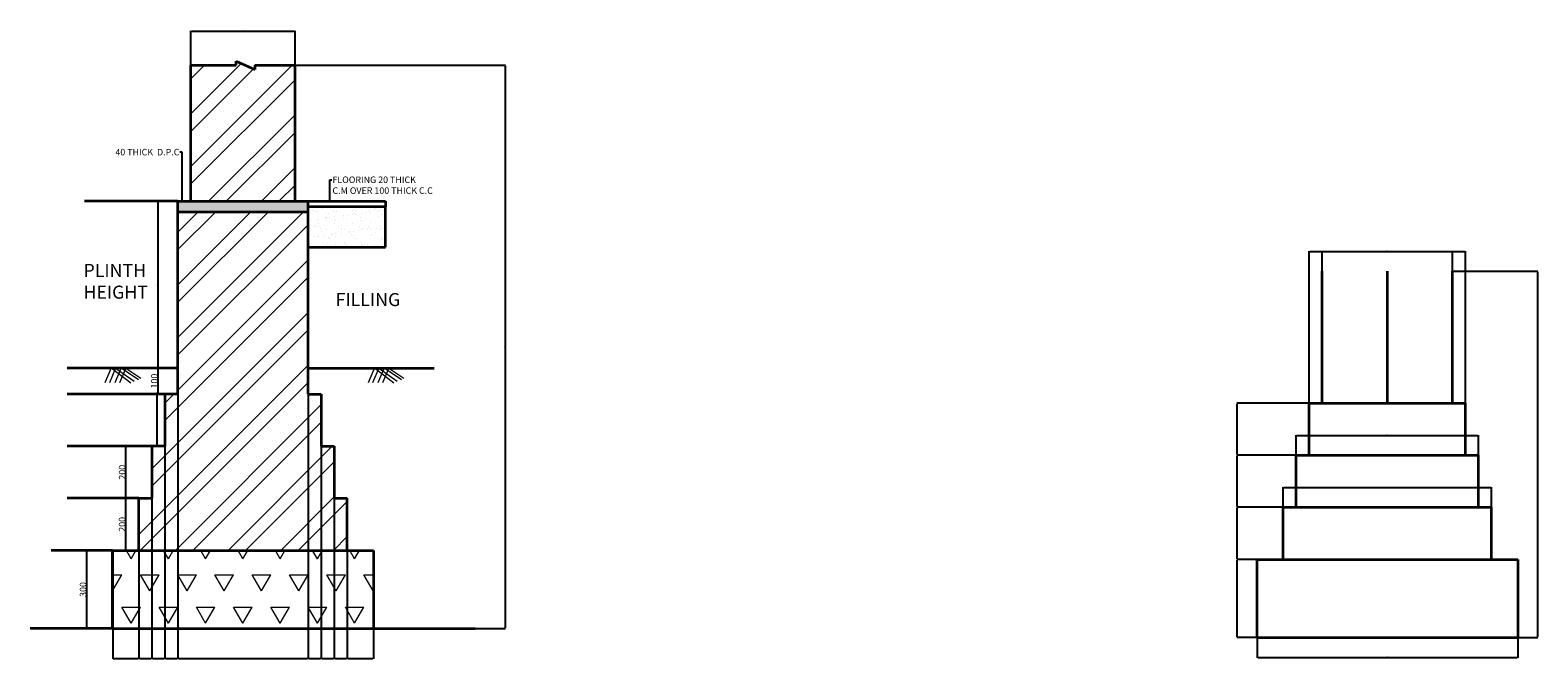
# Model space of a CAD drawing. Units: millimetres. Extents: x 31035 to 42175, y 1348 to 3924.
# Tile 2 of 2: x 36392 to 42175, y 1348 to 3761. Entities that reach past the tile are written whole.
import ezdxf
from ezdxf import colors
from ezdxf.entities.mleader import LeaderData, LeaderLine
from ezdxf.math import Vec2, Vec3

# ---------------------------------------------------------------- set-up
doc = ezdxf.new("R2010")
doc.units = ezdxf.units.MM
for name, color, linetype, lineweight in [('A-ANNO-DIMS', 2, 'Continuous', 18), ('A-ANNO-SYMB', 3, 'Continuous', 18), ('A-ANNO-TEXT', 7, 'Continuous', 18), ('A-SECT', 7, 'Continuous', 35), ('A-WALL-PATT', 8, 'Continuous', 13), ('C-TOPO-PATT', 9, 'Continuous', 13), ('S-FNDN-PATT', 252, 'Continuous', 13)]:
    doc.layers.add(name, color=color, linetype=linetype, lineweight=lineweight)
doc.styles.get("Standard").update_dxf_attribs({"font": 'arial.ttf'})
doc.dimstyles.new('ISO-25', dxfattribs={"dimtxt": 2.5, "dimasz": 2.5, "dimexe": 1.25, "dimexo": 0.625, "dimtad": 1, "dimtxsty": 'Standard', "dimcen": 2.5, "dimadec": 0, "dimazin": 0, "dimtfac": 1, "dimtmove": 0, "dimatfit": 3, "dimfxl": 1, "dimarcsym": 0})
pattern_1 = [(45, (28921.22, 0), (-101.0279, 101.0279), []), (45, (28988.58, 0), (-101.0279, 101.0279), [])]

# ---------------------------------------------------------------- blocks, each defined once
blk = doc.blocks.new('*D15')
at = {"layer": 'A-ANNO-DIMS', "color": 0, "lineweight": -2, "transparency": 16777216}
for p, q in [((36828.2, 3104.1), (36882.5, 3104.1)), ((36881.2, 3101.6), (36881.2, 2466.6)), ((36828.2, 2464.1), (36882.5, 2464.1))]:
    blk.add_line(p, q, dxfattribs=at)
at = {"layer": 'A-ANNO-DIMS', "color": 0, "transparency": 16777216}
for points in [[(36880.8, 3101.6), (36881.7, 3101.6), (36881.2, 3104.1)], [(36880.8, 2466.6), (36881.7, 2466.6), (36881.2, 2464.1)]]:
    blk.add_solid(points, dxfattribs=at)
at = {"layer": 'Defpoints', "color": 0, "transparency": 16777216}
for p in [(36827.6, 3104.1), (36827.6, 2464.1), (36881.2, 2464.1)]:
    blk.add_point(p, dxfattribs=at)
at = {"layer": 'A-ANNO-DIMS', "color": 0, "transparency": 16777216, "insert": (36879.3, 2784.1), "char_height": 2.5, "attachment_point": 5, "rotation": 90}
blk.add_mtext('640', dxfattribs=at)
blk = doc.blocks.new('*D16')
at = {"layer": 'A-ANNO-DIMS', "color": 0, "lineweight": -2, "transparency": 16777216}
for p, q in [((36881.4, 2461.6), (36881.4, 2366.6)), ((36881.9, 2464.1), (36882.7, 2464.1)), ((36881.9, 2364.1), (36882.7, 2364.1))]:
    blk.add_line(p, q, dxfattribs=at)
at = {"layer": 'A-ANNO-DIMS', "color": 0, "transparency": 16777216}
for points in [[(36881, 2461.6), (36881.9, 2461.6), (36881.4, 2464.1)], [(36881, 2366.6), (36881.9, 2366.6), (36881.4, 2364.1)]]:
    blk.add_solid(points, dxfattribs=at)
at = {"layer": 'Defpoints', "color": 0, "transparency": 16777216}
for p in [(36881.2, 2464.1), (36881.2, 2364.1), (36881.4, 2364.1)]:
    blk.add_point(p, dxfattribs=at)
at = {"layer": 'A-ANNO-DIMS', "color": 0, "transparency": 16777216, "insert": (36868.1, 2414.1), "char_height": 2.5, "attachment_point": 5, "rotation": 90}
blk.add_mtext('{\\H10x;100}', dxfattribs=at)
blk = doc.blocks.new('*D17')
at = {"layer": 'A-ANNO-DIMS', "color": 0, "lineweight": -2, "transparency": 16777216}
for p, q in [((36881.2, 2366.6), (36876.9, 2366.6)), ((36878.2, 2364.1), (36878.2, 2166.6)), ((36881.2, 2164.1), (36876.9, 2164.1))]:
    blk.add_line(p, q, dxfattribs=at)
at = {"layer": 'A-ANNO-DIMS', "color": 0, "transparency": 16777216}
for points in [[(36877.7, 2364.1), (36878.6, 2364.1), (36878.2, 2366.6)], [(36877.7, 2166.6), (36878.6, 2166.6), (36878.2, 2164.1)]]:
    blk.add_solid(points, dxfattribs=at)
at = {"layer": 'Defpoints', "color": 0, "transparency": 16777216}
for p in [(36881.9, 2366.6), (36878.2, 2164.1), (36881.9, 2164.1)]:
    blk.add_point(p, dxfattribs=at)
at = {"layer": 'A-ANNO-DIMS', "color": 0, "transparency": 16777216, "insert": (36876, 2265.3), "char_height": 2.5, "attachment_point": 5, "rotation": 90}
blk.add_mtext('202,5', dxfattribs=at)
blk = doc.blocks.new('*D18')
at = {"layer": 'A-ANNO-DIMS', "color": 0, "lineweight": -2, "transparency": 16777216}
for p, q in [((36758.3, 2161.6), (36758.3, 1966.6)), ((36758.9, 2164.1), (36759.5, 2164.1)), ((36758.9, 1964.1), (36759.5, 1964.1))]:
    blk.add_line(p, q, dxfattribs=at)
at = {"layer": 'A-ANNO-DIMS', "color": 0, "transparency": 16777216}
for points in [[(36757.8, 2161.6), (36758.7, 2161.6), (36758.3, 2164.1)], [(36757.8, 1966.6), (36758.7, 1966.6), (36758.3, 1964.1)]]:
    blk.add_solid(points, dxfattribs=at)
at = {"layer": 'Defpoints', "color": 0, "transparency": 16777216}
for p in [(36758.3, 2164.1), (36758.3, 1964.1), (36758.3, 1964.1)]:
    blk.add_point(p, dxfattribs=at)
at = {"layer": 'A-ANNO-DIMS', "color": 0, "transparency": 16777216, "insert": (36744.9, 2064.1), "char_height": 2.5, "attachment_point": 5, "rotation": 90}
blk.add_mtext('{\\H10x;200}', dxfattribs=at)
blk = doc.blocks.new('*D19')
at = {"layer": 'A-ANNO-DIMS', "color": 0, "lineweight": -2, "transparency": 16777216}
for p, q in [((36758.9, 1964.1), (36757, 1964.1)), ((36758.2, 1961.6), (36758.2, 1766.6)), ((36758.9, 1764.1), (36757, 1764.1))]:
    blk.add_line(p, q, dxfattribs=at)
at = {"layer": 'A-ANNO-DIMS', "color": 0, "transparency": 16777216}
for points in [[(36757.8, 1961.6), (36758.6, 1961.6), (36758.2, 1964.1)], [(36757.8, 1766.6), (36758.6, 1766.6), (36758.2, 1764.1)]]:
    blk.add_solid(points, dxfattribs=at)
at = {"layer": 'Defpoints', "color": 0, "transparency": 16777216}
for p in [(36759.5, 1964.1), (36758.2, 1764.1), (36759.5, 1764.1)]:
    blk.add_point(p, dxfattribs=at)
at = {"layer": 'A-ANNO-DIMS', "color": 0, "transparency": 16777216, "insert": (36744.8, 1864.1), "char_height": 2.5, "attachment_point": 5, "rotation": 90}
blk.add_mtext('{\\H10x;200}', dxfattribs=at)
blk = doc.blocks.new('*D20')
at = {"layer": 'A-ANNO-DIMS', "color": 0, "lineweight": -2, "transparency": 16777216}
for p, q in [((36631.4, 1764.1), (36607.1, 1764.1)), ((36608.3, 1761.6), (36608.3, 1466.6)), ((36631.4, 1464.1), (36607.1, 1464.1))]:
    blk.add_line(p, q, dxfattribs=at)
at = {"layer": 'A-ANNO-DIMS', "color": 0, "transparency": 16777216}
for points in [[(36607.9, 1761.6), (36608.7, 1761.6), (36608.3, 1764.1)], [(36607.9, 1466.6), (36608.7, 1466.6), (36608.3, 1464.1)]]:
    blk.add_solid(points, dxfattribs=at)
at = {"layer": 'Defpoints', "color": 0, "transparency": 16777216}
for p in [(36632, 1764.1), (36608.3, 1464.1), (36632, 1464.1)]:
    blk.add_point(p, dxfattribs=at)
at = {"layer": 'A-ANNO-DIMS', "color": 0, "transparency": 16777216, "insert": (36594.9, 1614.1), "char_height": 2.5, "attachment_point": 5, "rotation": 90}
blk.add_mtext('{\\H10x;300}', dxfattribs=at)
blk = doc.blocks.new('EARTH-SYMBOL-B')
for p, q in [((24.2, 58), (0, 0.7)), ((24.2, 58), (99.5, 0.7)), ((61.9, 58), (37.7, 0.7)), ((61.9, 58), (128.5, 13.8)), ((40.9, 57.3), (16.7, 0)), ((40.9, 57.3), (111.8, 6.5)), ((80.1, 57.3), (55.9, 0)), ((80.1, 57.3), (137.9, 18.1))]:
    blk.add_line(p, q)
blk = doc.blocks.new('*D26')
at = {"layer": 'A-ANNO-DIMS', "color": 0, "lineweight": -2, "transparency": 16777216}
for p, q in [((37409.1, 3626.5), (38214.9, 3626.5)), ((38213.7, 3624), (38213.7, 1466.6)), ((37709.1, 1464.1), (38214.9, 1464.1))]:
    blk.add_line(p, q, dxfattribs=at)
at = {"layer": 'A-ANNO-DIMS', "color": 0, "transparency": 16777216}
for points in [[(38213.3, 3624), (38214.1, 3624), (38213.7, 3626.5)], [(38213.3, 1466.6), (38214.1, 1466.6), (38213.7, 1464.1)]]:
    blk.add_solid(points, dxfattribs=at)
at = {"layer": 'Defpoints', "color": 0, "transparency": 16777216}
for p in [(37408.5, 3626.5), (37708.5, 1464.1), (38213.7, 1464.1)]:
    blk.add_point(p, dxfattribs=at)
at = {"layer": 'A-ANNO-DIMS', "color": 0, "transparency": 16777216, "insert": (38211.8, 2545.3), "char_height": 2.5, "attachment_point": 5, "rotation": 90}
blk.add_mtext('2162.4', dxfattribs=at)
blk = doc.blocks.new('*D27')
at = {"layer": 'A-ANNO-DIMS', "color": 0, "lineweight": -2, "transparency": 16777216}
for p, q in [((37008.5, 3627.2), (37008.5, 3758.8)), ((37011, 3757.5), (37406, 3757.5)), ((37408.5, 3627.2), (37408.5, 3758.8))]:
    blk.add_line(p, q, dxfattribs=at)
at = {"layer": 'A-ANNO-DIMS', "color": 0, "transparency": 16777216}
for points in [[(37011, 3757.9), (37011, 3757.1), (37008.5, 3757.5)], [(37406, 3757.9), (37406, 3757.1), (37408.5, 3757.5)]]:
    blk.add_solid(points, dxfattribs=at)
at = {"layer": 'Defpoints', "color": 0, "transparency": 16777216}
for p in [(37408.5, 3757.5), (37008.5, 3626.5), (37408.5, 3626.5)]:
    blk.add_point(p, dxfattribs=at)
at = {"layer": 'A-ANNO-DIMS', "color": 0, "transparency": 16777216, "insert": (37208.5, 3759.4), "char_height": 2.5, "attachment_point": 5}
blk.add_mtext('400', dxfattribs=at)
blk = doc.blocks.new('*D28')
at = {"layer": 'A-ANNO-DIMS', "color": 0, "lineweight": -2, "transparency": 16777216}
for p, q in [((41098.1, 1429), (41098.1, 1352.4)), ((42098.1, 1429), (42098.1, 1352.4)), ((41100.6, 1353.6), (42095.6, 1353.6))]:
    blk.add_line(p, q, dxfattribs=at)
at = {"layer": 'A-ANNO-DIMS', "color": 0, "transparency": 16777216}
for points in [[(41100.6, 1354.1), (41100.6, 1353.2), (41098.1, 1353.6)], [(42095.6, 1354.1), (42095.6, 1353.2), (42098.1, 1353.6)]]:
    blk.add_solid(points, dxfattribs=at)
at = {"layer": 'Defpoints', "color": 0, "transparency": 16777216}
for p in [(41098.1, 1429.6), (42098.1, 1429.6), (42098.1, 1353.6)]:
    blk.add_point(p, dxfattribs=at)
at = {"layer": 'A-ANNO-DIMS', "color": 0, "transparency": 16777216, "insert": (41598.1, 1355.5), "char_height": 2.5, "attachment_point": 5}
blk.add_mtext('1000', dxfattribs=at)
blk = doc.blocks.new('*D29')
at = {"layer": 'A-ANNO-DIMS', "color": 0, "lineweight": -2, "transparency": 16777216}
for p, q in [((41348.1, 2836.6), (41348.1, 2913.2)), ((41350.6, 2911.9), (41845.6, 2911.9)), ((41848.1, 2836.6), (41848.1, 2913.2))]:
    blk.add_line(p, q, dxfattribs=at)
at = {"layer": 'A-ANNO-DIMS', "color": 0, "transparency": 16777216}
for points in [[(41350.6, 2912.3), (41350.6, 2911.5), (41348.1, 2911.9)], [(41845.6, 2912.3), (41845.6, 2911.5), (41848.1, 2911.9)]]:
    blk.add_solid(points, dxfattribs=at)
at = {"layer": 'Defpoints', "color": 0, "transparency": 16777216}
for p in [(41848.1, 2911.9), (41348.1, 2835.9), (41848.1, 2835.9)]:
    blk.add_point(p, dxfattribs=at)
at = {"layer": 'A-ANNO-DIMS', "color": 0, "transparency": 16777216, "insert": (41598.1, 2913.8), "char_height": 2.5, "attachment_point": 5}
blk.add_mtext('500', dxfattribs=at)
blk = doc.blocks.new('*D30')
at = {"layer": 'A-ANNO-DIMS', "color": 0, "lineweight": -2, "transparency": 16777216}
for p, q in [((41097.5, 1729.6), (41020.8, 1729.6)), ((41022.1, 1432.1), (41022.1, 1727.1)), ((41097.5, 1429.6), (41020.8, 1429.6))]:
    blk.add_line(p, q, dxfattribs=at)
at = {"layer": 'A-ANNO-DIMS', "color": 0, "transparency": 16777216}
for points in [[(41021.7, 1727.1), (41022.5, 1727.1), (41022.1, 1729.6)], [(41021.7, 1432.1), (41022.5, 1432.1), (41022.1, 1429.6)]]:
    blk.add_solid(points, dxfattribs=at)
at = {"layer": 'Defpoints', "color": 0, "transparency": 16777216}
for p in [(41022.1, 1729.6), (41098.1, 1729.6), (41098.1, 1429.6)]:
    blk.add_point(p, dxfattribs=at)
at = {"layer": 'A-ANNO-DIMS', "color": 0, "transparency": 16777216, "insert": (41020.2, 1579.6), "char_height": 2.5, "attachment_point": 5, "rotation": 90}
blk.add_mtext('300', dxfattribs=at)
blk = doc.blocks.new('*D31')
at = {"layer": 'A-ANNO-DIMS', "color": 0, "lineweight": -2, "transparency": 16777216}
for p, q in [((41197.5, 1929.6), (41020.8, 1929.6)), ((41022.1, 1732.1), (41022.1, 1927.1)), ((41197.5, 1729.6), (41020.8, 1729.6))]:
    blk.add_line(p, q, dxfattribs=at)
at = {"layer": 'A-ANNO-DIMS', "color": 0, "transparency": 16777216}
for points in [[(41021.7, 1927.1), (41022.5, 1927.1), (41022.1, 1929.6)], [(41021.7, 1732.1), (41022.5, 1732.1), (41022.1, 1729.6)]]:
    blk.add_solid(points, dxfattribs=at)
at = {"layer": 'Defpoints', "color": 0, "transparency": 16777216}
for p in [(41022.1, 1929.6), (41198.1, 1929.6), (41198.1, 1729.6)]:
    blk.add_point(p, dxfattribs=at)
at = {"layer": 'A-ANNO-DIMS', "color": 0, "transparency": 16777216, "insert": (41020.2, 1829.6), "char_height": 2.5, "attachment_point": 5, "rotation": 90}
blk.add_mtext('200', dxfattribs=at)
blk = doc.blocks.new('*D32')
at = {"layer": 'A-ANNO-DIMS', "color": 0, "lineweight": -2, "transparency": 16777216}
for p, q in [((41247.5, 2129.6), (41020.8, 2129.6)), ((41022.1, 1932.1), (41022.1, 2127.1)), ((41247.5, 1929.6), (41020.8, 1929.6))]:
    blk.add_line(p, q, dxfattribs=at)
at = {"layer": 'A-ANNO-DIMS', "color": 0, "transparency": 16777216}
for points in [[(41021.7, 2127.1), (41022.5, 2127.1), (41022.1, 2129.6)], [(41021.7, 1932.1), (41022.5, 1932.1), (41022.1, 1929.6)]]:
    blk.add_solid(points, dxfattribs=at)
at = {"layer": 'Defpoints', "color": 0, "transparency": 16777216}
for p in [(41022.1, 2129.6), (41248.1, 2129.6), (41248.1, 1929.6)]:
    blk.add_point(p, dxfattribs=at)
at = {"layer": 'A-ANNO-DIMS', "color": 0, "transparency": 16777216, "insert": (41020.2, 2029.6), "char_height": 2.5, "attachment_point": 5, "rotation": 90}
blk.add_mtext('200', dxfattribs=at)
blk = doc.blocks.new('*D33')
at = {"layer": 'A-ANNO-DIMS', "color": 0, "lineweight": -2, "transparency": 16777216}
for p, q in [((41297.5, 2329.6), (41020.8, 2329.6)), ((41022.1, 2132.1), (41022.1, 2327.1)), ((41297.5, 2129.6), (41020.8, 2129.6))]:
    blk.add_line(p, q, dxfattribs=at)
at = {"layer": 'A-ANNO-DIMS', "color": 0, "transparency": 16777216}
for points in [[(41021.7, 2327.1), (41022.5, 2327.1), (41022.1, 2329.6)], [(41021.7, 2132.1), (41022.5, 2132.1), (41022.1, 2129.6)]]:
    blk.add_solid(points, dxfattribs=at)
at = {"layer": 'Defpoints', "color": 0, "transparency": 16777216}
for p in [(41022.1, 2329.6), (41298.1, 2329.6), (41298.1, 2129.6)]:
    blk.add_point(p, dxfattribs=at)
at = {"layer": 'A-ANNO-DIMS', "color": 0, "transparency": 16777216, "insert": (41020.2, 2229.6), "char_height": 2.5, "attachment_point": 5, "rotation": 90}
blk.add_mtext('200', dxfattribs=at)
blk = doc.blocks.new('*D34')
at = {"layer": 'A-ANNO-DIMS', "color": 0, "lineweight": -2, "transparency": 16777216}
for p, q in [((41198.1, 1930.3), (41198.1, 2006.9)), ((41200.6, 2005.6), (41995.6, 2005.6)), ((41998.1, 1930.3), (41998.1, 2006.9))]:
    blk.add_line(p, q, dxfattribs=at)
at = {"layer": 'A-ANNO-DIMS', "color": 0, "transparency": 16777216}
for points in [[(41200.6, 2006.1), (41200.6, 2005.2), (41198.1, 2005.6)], [(41995.6, 2006.1), (41995.6, 2005.2), (41998.1, 2005.6)]]:
    blk.add_solid(points, dxfattribs=at)
at = {"layer": 'Defpoints', "color": 0, "transparency": 16777216}
for p in [(41998.1, 2005.6), (41198.1, 1929.6), (41998.1, 1929.6)]:
    blk.add_point(p, dxfattribs=at)
at = {"layer": 'A-ANNO-DIMS', "color": 0, "transparency": 16777216, "insert": (41598.1, 2007.5), "char_height": 2.5, "attachment_point": 5}
blk.add_mtext('800', dxfattribs=at)
blk = doc.blocks.new('*D35')
at = {"layer": 'A-ANNO-DIMS', "color": 0, "lineweight": -2, "transparency": 16777216}
for p, q in [((41248.1, 2130.3), (41248.1, 2206.9)), ((41250.6, 2205.6), (41945.6, 2205.6)), ((41948.1, 2130.3), (41948.1, 2206.9))]:
    blk.add_line(p, q, dxfattribs=at)
at = {"layer": 'A-ANNO-DIMS', "color": 0, "transparency": 16777216}
for points in [[(41250.6, 2206.1), (41250.6, 2205.2), (41248.1, 2205.6)], [(41945.6, 2206.1), (41945.6, 2205.2), (41948.1, 2205.6)]]:
    blk.add_solid(points, dxfattribs=at)
at = {"layer": 'Defpoints', "color": 0, "transparency": 16777216}
for p in [(41948.1, 2205.6), (41248.1, 2129.6), (41948.1, 2129.6)]:
    blk.add_point(p, dxfattribs=at)
at = {"layer": 'A-ANNO-DIMS', "color": 0, "transparency": 16777216, "insert": (41598.1, 2207.5), "char_height": 2.5, "attachment_point": 5}
blk.add_mtext('700', dxfattribs=at)
blk = doc.blocks.new('*D36')
at = {"layer": 'A-ANNO-DIMS', "color": 0, "lineweight": -2, "transparency": 16777216}
for p, q in [((41298.1, 2330.3), (41298.1, 2913.2)), ((41300.6, 2911.9), (41895.6, 2911.9)), ((41898.1, 2330.3), (41898.1, 2913.2))]:
    blk.add_line(p, q, dxfattribs=at)
at = {"layer": 'A-ANNO-DIMS', "color": 0, "transparency": 16777216}
for points in [[(41300.6, 2912.3), (41300.6, 2911.5), (41298.1, 2911.9)], [(41895.6, 2912.3), (41895.6, 2911.5), (41898.1, 2911.9)]]:
    blk.add_solid(points, dxfattribs=at)
at = {"layer": 'Defpoints', "color": 0, "transparency": 16777216}
for p in [(41898.1, 2911.9), (41298.1, 2329.6), (41898.1, 2329.6)]:
    blk.add_point(p, dxfattribs=at)
at = {"layer": 'A-ANNO-DIMS', "color": 0, "transparency": 16777216, "insert": (41598.1, 2913.8), "char_height": 2.5, "attachment_point": 5}
blk.add_mtext('600', dxfattribs=at)
blk = doc.blocks.new('*D37')
at = {"layer": 'A-ANNO-DIMS', "color": 0, "lineweight": -2, "transparency": 16777216}
for p, q in [((41848.7, 2835.9), (42175.3, 2835.9)), ((42174.1, 2833.4), (42174.1, 1432.1)), ((42098.7, 1429.6), (42175.3, 1429.6))]:
    blk.add_line(p, q, dxfattribs=at)
at = {"layer": 'A-ANNO-DIMS', "color": 0, "transparency": 16777216}
for points in [[(42173.7, 2833.4), (42174.5, 2833.4), (42174.1, 2835.9)], [(42173.7, 1432.1), (42174.5, 1432.1), (42174.1, 1429.6)]]:
    blk.add_solid(points, dxfattribs=at)
at = {"layer": 'Defpoints', "color": 0, "transparency": 16777216}
for p in [(41848.1, 2835.9), (42098.1, 1429.6), (42174.1, 1429.6)]:
    blk.add_point(p, dxfattribs=at)
at = {"layer": 'A-ANNO-DIMS', "color": 0, "transparency": 16777216, "insert": (42172.2, 2132.8), "char_height": 2.5, "attachment_point": 5, "rotation": 90}
blk.add_mtext('1406.3', dxfattribs=at)
blk = doc.blocks.new('*D45')
at = {"layer": 'A-ANNO-DIMS', "color": 0, "lineweight": -2, "transparency": 16777216}
for p, q in [((36708.5, 1763.5), (36708.5, 1347.8)), ((36808.5, 1763.5), (36808.5, 1347.8)), ((36711, 1349.1), (36806, 1349.1))]:
    blk.add_line(p, q, dxfattribs=at)
at = {"layer": 'A-ANNO-DIMS', "color": 0, "transparency": 16777216}
for points in [[(36711, 1349.5), (36711, 1348.7), (36708.5, 1349.1)], [(36806, 1349.5), (36806, 1348.7), (36808.5, 1349.1)]]:
    blk.add_solid(points, dxfattribs=at)
at = {"layer": 'Defpoints', "color": 0, "transparency": 16777216}
for p in [(36708.5, 1764.1), (36808.5, 1764.1), (36808.5, 1349.1)]:
    blk.add_point(p, dxfattribs=at)
at = {"layer": 'A-ANNO-DIMS', "color": 0, "transparency": 16777216, "insert": (36758.5, 1351), "char_height": 2.5, "attachment_point": 5}
blk.add_mtext('100', dxfattribs=at)
blk = doc.blocks.new('*D46')
at = {"layer": 'A-ANNO-DIMS', "color": 0, "lineweight": -2, "transparency": 16777216}
for p, q in [((36858.5, 1963.5), (36858.5, 1347.8)), ((36808.5, 1763.5), (36808.5, 1347.8)), ((36811, 1349.1), (36856, 1349.1))]:
    blk.add_line(p, q, dxfattribs=at)
at = {"layer": 'A-ANNO-DIMS', "color": 0, "transparency": 16777216}
for points in [[(36811, 1349.5), (36811, 1348.7), (36808.5, 1349.1)], [(36856, 1349.5), (36856, 1348.7), (36858.5, 1349.1)]]:
    blk.add_solid(points, dxfattribs=at)
at = {"layer": 'Defpoints', "color": 0, "transparency": 16777216}
for p in [(36858.5, 1964.1), (36808.5, 1764.1), (36858.5, 1349.1)]:
    blk.add_point(p, dxfattribs=at)
at = {"layer": 'A-ANNO-DIMS', "color": 0, "transparency": 16777216, "insert": (36833.5, 1351), "char_height": 2.5, "attachment_point": 5}
blk.add_mtext('50', dxfattribs=at)
blk = doc.blocks.new('*D47')
at = {"layer": 'A-ANNO-DIMS', "color": 0, "lineweight": -2, "transparency": 16777216}
for p, q in [((36908.5, 2163.5), (36908.5, 1347.8)), ((36858.5, 1963.5), (36858.5, 1347.8)), ((36861, 1349.1), (36906, 1349.1))]:
    blk.add_line(p, q, dxfattribs=at)
at = {"layer": 'A-ANNO-DIMS', "color": 0, "transparency": 16777216}
for points in [[(36861, 1349.5), (36861, 1348.7), (36858.5, 1349.1)], [(36906, 1349.5), (36906, 1348.7), (36908.5, 1349.1)]]:
    blk.add_solid(points, dxfattribs=at)
at = {"layer": 'Defpoints', "color": 0, "transparency": 16777216}
for p in [(36908.5, 2164.1), (36858.5, 1964.1), (36908.5, 1349.1)]:
    blk.add_point(p, dxfattribs=at)
at = {"layer": 'A-ANNO-DIMS', "color": 0, "transparency": 16777216, "insert": (36883.5, 1351), "char_height": 2.5, "attachment_point": 5}
blk.add_mtext('50', dxfattribs=at)
blk = doc.blocks.new('*D48')
at = {"layer": 'A-ANNO-DIMS', "color": 0, "lineweight": -2, "transparency": 16777216}
for p, q in [((36958.5, 2363.5), (36958.5, 1347.8)), ((36908.5, 2163.5), (36908.5, 1347.8)), ((36911, 1349.1), (36956, 1349.1))]:
    blk.add_line(p, q, dxfattribs=at)
at = {"layer": 'A-ANNO-DIMS', "color": 0, "transparency": 16777216}
for points in [[(36911, 1349.5), (36911, 1348.7), (36908.5, 1349.1)], [(36956, 1349.5), (36956, 1348.7), (36958.5, 1349.1)]]:
    blk.add_solid(points, dxfattribs=at)
at = {"layer": 'Defpoints', "color": 0, "transparency": 16777216}
for p in [(36958.5, 2364.1), (36908.5, 2164.1), (36958.5, 1349.1)]:
    blk.add_point(p, dxfattribs=at)
at = {"layer": 'A-ANNO-DIMS', "color": 0, "transparency": 16777216, "insert": (36933.5, 1351), "char_height": 2.5, "attachment_point": 5}
blk.add_mtext('50', dxfattribs=at)
blk = doc.blocks.new('*D49')
at = {"layer": 'A-ANNO-DIMS', "color": 0, "lineweight": -2, "transparency": 16777216}
for p, q in [((36958.5, 2363.5), (36958.5, 1347.8)), ((37458.5, 2363.5), (37458.5, 1347.8)), ((36961, 1349.1), (37456, 1349.1))]:
    blk.add_line(p, q, dxfattribs=at)
at = {"layer": 'A-ANNO-DIMS', "color": 0, "transparency": 16777216}
for points in [[(36961, 1349.5), (36961, 1348.7), (36958.5, 1349.1)], [(37456, 1349.5), (37456, 1348.7), (37458.5, 1349.1)]]:
    blk.add_solid(points, dxfattribs=at)
at = {"layer": 'Defpoints', "color": 0, "transparency": 16777216}
for p in [(36958.5, 2364.1), (37458.5, 2364.1), (37458.5, 1349.1)]:
    blk.add_point(p, dxfattribs=at)
at = {"layer": 'A-ANNO-DIMS', "color": 0, "transparency": 16777216, "insert": (37208.5, 1351), "char_height": 2.5, "attachment_point": 5}
blk.add_mtext('500', dxfattribs=at)
blk = doc.blocks.new('*D50')
at = {"layer": 'A-ANNO-DIMS', "color": 0, "lineweight": -2, "transparency": 16777216}
for p, q in [((37458.5, 2363.5), (37458.5, 1347.8)), ((37508.5, 2163.5), (37508.5, 1347.8)), ((37461, 1349.1), (37506, 1349.1))]:
    blk.add_line(p, q, dxfattribs=at)
at = {"layer": 'A-ANNO-DIMS', "color": 0, "transparency": 16777216}
for points in [[(37461, 1349.5), (37461, 1348.7), (37458.5, 1349.1)], [(37506, 1349.5), (37506, 1348.7), (37508.5, 1349.1)]]:
    blk.add_solid(points, dxfattribs=at)
at = {"layer": 'Defpoints', "color": 0, "transparency": 16777216}
for p in [(37458.5, 2364.1), (37508.5, 2164.1), (37508.5, 1349.1)]:
    blk.add_point(p, dxfattribs=at)
at = {"layer": 'A-ANNO-DIMS', "color": 0, "transparency": 16777216, "insert": (37483.5, 1351), "char_height": 2.5, "attachment_point": 5}
blk.add_mtext('50', dxfattribs=at)
blk = doc.blocks.new('*D51')
at = {"layer": 'A-ANNO-DIMS', "color": 0, "lineweight": -2, "transparency": 16777216}
for p, q in [((37508.5, 2163.5), (37508.5, 1347.8)), ((37558.5, 1963.5), (37558.5, 1347.8)), ((37511, 1349.1), (37556, 1349.1))]:
    blk.add_line(p, q, dxfattribs=at)
at = {"layer": 'A-ANNO-DIMS', "color": 0, "transparency": 16777216}
for points in [[(37511, 1349.5), (37511, 1348.7), (37508.5, 1349.1)], [(37556, 1349.5), (37556, 1348.7), (37558.5, 1349.1)]]:
    blk.add_solid(points, dxfattribs=at)
at = {"layer": 'Defpoints', "color": 0, "transparency": 16777216}
for p in [(37508.5, 2164.1), (37558.5, 1964.1), (37558.5, 1349.1)]:
    blk.add_point(p, dxfattribs=at)
at = {"layer": 'A-ANNO-DIMS', "color": 0, "transparency": 16777216, "insert": (37533.5, 1351), "char_height": 2.5, "attachment_point": 5}
blk.add_mtext('50', dxfattribs=at)
blk = doc.blocks.new('*D52')
at = {"layer": 'A-ANNO-DIMS', "color": 0, "lineweight": -2, "transparency": 16777216}
for p, q in [((37558.5, 1963.5), (37558.5, 1347.8)), ((37608.5, 1763.5), (37608.5, 1347.8)), ((37561, 1349.1), (37606, 1349.1))]:
    blk.add_line(p, q, dxfattribs=at)
at = {"layer": 'A-ANNO-DIMS', "color": 0, "transparency": 16777216}
for points in [[(37561, 1349.5), (37561, 1348.7), (37558.5, 1349.1)], [(37606, 1349.5), (37606, 1348.7), (37608.5, 1349.1)]]:
    blk.add_solid(points, dxfattribs=at)
at = {"layer": 'Defpoints', "color": 0, "transparency": 16777216}
for p in [(37558.5, 1964.1), (37608.5, 1764.1), (37608.5, 1349.1)]:
    blk.add_point(p, dxfattribs=at)
at = {"layer": 'A-ANNO-DIMS', "color": 0, "transparency": 16777216, "insert": (37583.5, 1351), "char_height": 2.5, "attachment_point": 5}
blk.add_mtext('50', dxfattribs=at)
blk = doc.blocks.new('*D53')
at = {"layer": 'A-ANNO-DIMS', "color": 0, "lineweight": -2, "transparency": 16777216}
for p, q in [((37608.5, 1763.5), (37608.5, 1347.8)), ((37708.5, 1763.5), (37708.5, 1347.8)), ((37611, 1349.1), (37706, 1349.1))]:
    blk.add_line(p, q, dxfattribs=at)
at = {"layer": 'A-ANNO-DIMS', "color": 0, "transparency": 16777216}
for points in [[(37611, 1349.5), (37611, 1348.7), (37608.5, 1349.1)], [(37706, 1349.5), (37706, 1348.7), (37708.5, 1349.1)]]:
    blk.add_solid(points, dxfattribs=at)
at = {"layer": 'Defpoints', "color": 0, "transparency": 16777216}
for p in [(37608.5, 1764.1), (37708.5, 1764.1), (37708.5, 1349.1)]:
    blk.add_point(p, dxfattribs=at)
at = {"layer": 'A-ANNO-DIMS', "color": 0, "transparency": 16777216, "insert": (37658.5, 1351), "char_height": 2.5, "attachment_point": 5}
blk.add_mtext('100', dxfattribs=at)

msp = doc.modelspace()

# ---------------------------------------------------------------- hatches: boundary and pattern name
at = {"layer": 'A-WALL-PATT'}
h = msp.add_hatch(dxfattribs=at)
h.set_pattern_fill('ANSI32', color=256, scale=15)
h.set_pattern_definition(pattern_1)
h.paths.add_polyline_path([(37408.462, 3626.533), (37253.522, 3626.533), (37253.522, 3610.438), (37182.554, 3642.505), (37182.554, 3626.533), (37008.462, 3626.533), (37008.462, 3104.085), (37408.462, 3104.085)])
h = msp.add_hatch(color=256, dxfattribs=at)
h.dxf.hatch_style = 1
h.paths.add_polyline_path([(37458.462, 3104.085), (36958.462, 3104.085), (36958.462, 3064.085), (37458.462, 3064.085)])
h = msp.add_hatch(dxfattribs=at)
h.set_pattern_fill('ANSI32', color=256, scale=15)
h.set_pattern_definition(pattern_1)
h.paths.add_polyline_path([(37458.462, 3064.085), (36958.462, 3064.085), (36958.462, 2364.085), (36908.462, 2364.085), (36908.462, 2164.085), (36858.462, 2164.085), (36858.462, 1964.085), (36808.462, 1964.085), (36808.462, 1764.085), (37608.462, 1764.085), (37608.462, 1964.085), (37558.462, 1964.085), (37558.462, 2164.085), (37508.462, 2164.085), (37508.462, 2364.085), (37458.462, 2364.085)])
at = {"layer": 'C-TOPO-PATT'}
h = msp.add_hatch(dxfattribs=at)
h.set_pattern_fill('AR-SAND', color=256)
h.set_pattern_definition([(37.5, (28921.223, 0), (-1.60003, 48.94132), [0, -38.608, 0, -43.18, 0, -41.275]), (7.5, (28921.223, 0), (44.95233, 71.6825), [0, -20.828, 0, -34.798, 0, -13.335]), (327.5, (28889.98, 0), (79.09924, 0.14372), [0, -12.7, 0, -45.72, 0, -59.69]), (317.5, (28889.98, 0), (76.35565, 22.29293), [0, -6.35, 0, -29.972, 0, -34.29])])
h.paths.add_polyline_path([(37755.169, 2928.49), (37755.169, 3084.085), (37458.462, 3084.085), (37458.462, 2928.49)])
at = {"layer": 'S-FNDN-PATT'}
h = msp.add_hatch(dxfattribs=at)
h.set_pattern_fill('TRIANG', color=256, scale=15)
h.set_pattern_definition([(60, (28921.22, 0), (-71.4375, 123.7334), [71.4375, -71.4375]), (120, (28921.22, 0), (-142.875, 8e-08), [71.4375, -71.4375]), (0, (28885.5, 61.87), (71.4375, 123.7334), [71.4375, -71.4375])])
h.paths.add_polyline_path([(36708.462, 1764.085), (36708.462, 1464.085), (37708.462, 1464.085), (37708.462, 1764.085)])

# ---------------------------------------------------------------- linework, layer by layer
at = {"layer": 'A-SECT'}
for p, q in [((37008.462, 3104.085), (37008.462, 3626.533)), ((37008.462, 3626.533), (37182.554, 3626.533)), ((37182.554, 3642.505), (37253.522, 3610.438)), ((37253.522, 3626.533), (37408.462, 3626.533)), ((37408.462, 3104.085), (37408.462, 3626.533)), ((36958.462, 3104.085), (36600.608, 3104.085)), ((36958.462, 2364.085), (36958.462, 3104.085)), ((36958.462, 3104.085), (37458.462, 3104.085)), ((37458.462, 2364.085), (37458.462, 3104.085)), ((37458.462, 3104.085), (37755.169, 3104.085)), ((37458.462, 3084.085), (37755.169, 3084.085)), ((37755.169, 3104.085), (37755.169, 3084.085)), ((37755.169, 2928.49), (37755.169, 3084.085)), ((36958.462, 3064.085), (37458.462, 3064.085)), ((37458.462, 2928.49), (37755.169, 2928.49)), ((41348.094, 2329.636), (41348.094, 2835.929)), ((41598.094, 2329.636), (41598.094, 2835.929)), ((41848.094, 2329.636), (41848.094, 2835.929)), ((36958.462, 2464.085), (36534.571, 2464.085)), ((37458.462, 2464.085), (37942.141, 2464.085)), ((36908.462, 2364.085), (36534.571, 2364.085)), ((36958.462, 2364.085), (36908.462, 2364.085)), ((36908.462, 2364.085), (36908.462, 2164.085)), ((37458.462, 2364.085), (37508.462, 2364.085)), ((37508.462, 2364.085), (37508.462, 2164.085)), ((41298.094, 2329.636), (41898.094, 2329.636)), ((41298.094, 2129.636), (41298.094, 2329.636)), ((41898.094, 2129.636), (41898.094, 2329.636)), ((36858.462, 2164.085), (36534.571, 2164.085)), ((36908.462, 2164.085), (36858.462, 2164.085)), ((36858.462, 2164.085), (36858.462, 1964.085)), ((37508.462, 2164.085), (37558.462, 2164.085)), ((37558.462, 2164.085), (37558.462, 1964.085)), ((41248.094, 2129.636), (41948.094, 2129.636)), ((41248.094, 1929.636), (41248.094, 2129.636)), ((41948.094, 1929.636), (41948.094, 2129.636)), ((36808.462, 1964.085), (36534.571, 1964.085)), ((36808.462, 1764.085), (36808.462, 1964.085)), ((36808.462, 1964.085), (36858.462, 1964.085)), ((37558.462, 1964.085), (37608.462, 1964.085)), ((37608.462, 1764.085), (37608.462, 1964.085)), ((41198.094, 1729.636), (41198.094, 1929.636)), ((41198.094, 1929.636), (41998.094, 1929.636)), ((41998.094, 1729.636), (41998.094, 1929.636)), ((36708.462, 1764.085), (36472.92, 1764.085)), ((36708.462, 1464.085), (36708.462, 1764.085)), ((36708.462, 1764.085), (37708.462, 1764.085)), ((37708.462, 1764.085), (37708.462, 1464.085)), ((41098.094, 1429.636), (41098.094, 1729.636)), ((41098.094, 1729.636), (42098.094, 1729.636)), ((42098.094, 1729.636), (42098.094, 1429.636)), ((36708.462, 1464.085), (36391.959, 1464.085)), ((36708.462, 1464.085), (37708.462, 1464.085)), ((37708.462, 1464.085), (38098.686, 1464.085)), ((41098.094, 1429.636), (42098.094, 1429.636))]:
    msp.add_line(p, q, dxfattribs=at)
for points in [[(37182.554, 3626.533), (37182.554, 3642.505)], [(37253.522, 3626.533), (37253.522, 3610.438)]]:
    msp.add_lwpolyline(points, dxfattribs=at)

# ---------------------------------------------------------------- block references
at = {"layer": 'A-ANNO-SYMB'}
for p in [(36679.062, 2406.793), (37688.064, 2406.793)]:
    msp.add_blockref('EARTH-SYMBOL-B', p, dxfattribs=at)

# ---------------------------------------------------------------- texts
at = {"layer": 'A-ANNO-TEXT', "char_height": 50, "attachment_point": 1}
for s, insert in [('PLINTH  HEIGHT ', (36596.542, 2863.732)), ('FILLING', (37563.845, 2751.778))]:
    msp.add_mtext_dynamic_manual_height_columns(s, width=135.33088, gutter_width=12.5, heights=[0], dxfattribs=dict(at, insert=insert))

# ---------------------------------------------------------------- dimensions: what is measured, and where the dimension line sits
at = {"layer": 'A-ANNO-DIMS'}
for base, p1, p2, picture, middle in [((37408.462, 3757.505), (37008.462, 3626.533), (37408.462, 3626.533), '*D27', (37208.462, 3759.407)), ((41898.094, 2911.929), (41298.094, 2329.636), (41898.094, 2329.636), '*D36', (41598.094, 2913.83)), ((41848.094, 2911.929), (41348.094, 2835.929), (41848.094, 2835.929), '*D29', (41598.094, 2913.83)), ((36958.462, 1349.085), (36908.462, 2164.085), (36958.462, 2364.085), '*D48', (36933.462, 1350.986)), ((37458.462, 1349.085), (36958.462, 2364.085), (37458.462, 2364.085), '*D49', (37208.462, 1350.986)), ((37508.462, 1349.085), (37458.462, 2364.085), (37508.462, 2164.085), '*D50', (37483.462, 1350.986)), ((41948.094, 2205.636), (41248.094, 2129.636), (41948.094, 2129.636), '*D35', (41598.094, 2207.538)), ((36908.462, 1349.085), (36858.462, 1964.085), (36908.462, 2164.085), '*D47', (36883.462, 1350.986)), ((37558.462, 1349.085), (37508.462, 2164.085), (37558.462, 1964.085), '*D51', (37533.462, 1350.986)), ((41998.094, 2005.636), (41198.094, 1929.636), (41998.094, 1929.636), '*D34', (41598.094, 2007.538)), ((36858.462, 1349.085), (36808.462, 1764.085), (36858.462, 1964.085), '*D46', (36833.462, 1350.986)), ((37608.462, 1349.085), (37558.462, 1964.085), (37608.462, 1764.085), '*D52', (37583.462, 1350.986)), ((36808.462, 1349.085), (36708.462, 1764.085), (36808.462, 1764.085), '*D45', (36758.462, 1350.986)), ((37708.462, 1349.085), (37608.462, 1764.085), (37708.462, 1764.085), '*D53', (37658.462, 1350.986)), ((42098.094, 1353.636), (41098.094, 1429.636), (42098.094, 1429.636), '*D28', (41598.094, 1355.538))]:
    dim = msp.add_linear_dim(base=base, p1=p1, p2=p2, dimstyle='ISO-25', override={"dimdec": 0, "dimlfac": 1, "dimrnd": 0, "dimzin": 0, "dimdsep": 46, "dimlunit": 2}, dxfattribs=at)
    dim.commit()
    dim.dimension.update_dxf_attribs({"geometry": picture, "text_midpoint": middle})
for base, p1, p2, override, picture, middle in [((38213.686, 1464.085), (37408.462, 3626.533), (37708.462, 1464.085), {"dimdec": 1, "dimlfac": 1, "dimrnd": 0, "dimzin": 0, "dimdsep": 46, "dimlunit": 2}, '*D26', (38211.784, 2545.309)), ((36881.234, 2464.085), (36827.56, 3104.085), (36827.56, 2464.085), {"dimclrd": 0, "dimclre": 0, "dimclrt": 0}, '*D15', (36879.333, 2784.085)), ((42174.094, 1429.636), (41848.094, 2835.929), (42098.094, 1429.636), {"dimdec": 1, "dimlfac": 1, "dimrnd": 0, "dimzin": 0, "dimdsep": 46, "dimlunit": 2}, '*D37', (42172.192, 2132.783)), ((36878.157, 2164.085), (36881.86, 2366.585), (36881.86, 2164.085), {"dimclrd": 0, "dimclre": 0, "dimclrt": 0}, '*D17', (36876.029, 2265.335)), ((41022.094, 2329.636), (41298.094, 2129.636), (41298.094, 2329.636), {"dimdec": 0, "dimlfac": 1, "dimrnd": 0, "dimzin": 0, "dimdsep": 46, "dimlunit": 2}, '*D33', (41020.193, 2229.636)), ((41022.094, 2129.636), (41248.094, 1929.636), (41248.094, 2129.636), {"dimdec": 0, "dimlfac": 1, "dimrnd": 0, "dimzin": 0, "dimdsep": 46, "dimlunit": 2}, '*D32', (41020.193, 2029.636)), ((41022.094, 1929.636), (41198.094, 1729.636), (41198.094, 1929.636), {"dimdec": 0, "dimlfac": 1, "dimrnd": 0, "dimzin": 0, "dimdsep": 46, "dimlunit": 2}, '*D31', (41020.193, 1829.636)), ((41022.094, 1729.636), (41098.094, 1429.636), (41098.094, 1729.636), {"dimdec": 0, "dimlfac": 1, "dimrnd": 0, "dimzin": 0, "dimdsep": 46, "dimlunit": 2}, '*D30', (41020.192, 1579.636))]:
    dim = msp.add_linear_dim(base=base, p1=p1, p2=p2, angle=90, dimstyle='ISO-25', override=override, dxfattribs=at)
    dim.commit()
    dim.dimension.update_dxf_attribs({"geometry": picture, "text_midpoint": middle})
for base, p1, p2, picture, middle in [((36881.443, 2364.085), (36881.234, 2464.085), (36881.234, 2364.085), '*D16', (36868.054, 2414.085)), ((36758.256, 1964.085), (36758.256, 2164.085), (36758.256, 1964.085), '*D18', (36744.867, 2064.085)), ((36758.223, 1764.085), (36759.506, 1964.085), (36759.506, 1764.085), '*D19', (36744.833, 1864.085)), ((36608.305, 1464.085), (36632.043, 1764.085), (36632.043, 1464.085), '*D20', (36594.907, 1614.085))]:
    dim = msp.add_linear_dim(base=base, p1=p1, p2=p2, angle=90, text='{\\H10x;<>}', dimstyle='ISO-25', override={"dimclrd": 0, "dimclre": 0, "dimclrt": 0}, dxfattribs=at)
    dim.commit()
    dim.dimension.update_dxf_attribs({"geometry": picture, "text_midpoint": middle})

# ---------------------------------------------------------------- leaders
at = {"layer": 'A-ANNO-TEXT'}
ml = msp.add_multileader_mtext('Standard', dxfattribs=at)
ml.set_content('40 THICK  D.P.C', color=256)
ml.set_leader_properties()
ml.build(insert=Vec2(0, 0))
ctx = ml.context
ctx.base_point, ctx.char_height, ctx.plane_origin = Vec3(36698.409, 3292.597), 25, Vec3(36974.461, 3104.085)
ctx.text_align_type = 2
notes = []
notes.append((ctx, [(0, (1, 1, 0), (36974.461, 3292.597), (-1, 0), 8, [(0, [(36974.461, 3104.085)], 0, [])])]))
ctx.mtext.insert, ctx.mtext.alignment, ctx.mtext.flow_direction = Vec3(36964.461, 3305.31), 3, 5
ml = msp.add_multileader_mtext('Standard', dxfattribs=at)
ml.set_content('FLOORING 20 THICK \\PC.M OVER 100 THICK C.C', color=256)
ml.set_leader_properties()
ml.build(insert=Vec2(0, 0))
ctx = ml.context
ctx.base_point, ctx.char_height, ctx.plane_origin = Vec3(37549.599, 3186.544), 25, Vec3(37541.599, 3101.111)
notes.append((ctx, [(0, (1, 1, 0), (37541.599, 3186.544), (1, 0), 8, [(0, [(37541.599, 3101.111)], 0, [])])]))
ctx.mtext.insert, ctx.mtext.flow_direction = Vec3(37551.599, 3199.258), 5
for ctx, leaders in notes:
    for number, flags, end, landing, length, lines in leaders:
        leader = LeaderData()
        leader.index, (leader.has_last_leader_line, leader.has_dogleg_vector, leader.attachment_direction) = number, flags
        leader.last_leader_point, leader.dogleg_vector, leader.dogleg_length = Vec3(end), Vec3(landing), length
        for number, points, colour, breaks in lines:
            line = LeaderLine()
            line.index, line.vertices, line.color, line.breaks = number, Vec3.list(points), colors.encode_raw_color(colour), breaks
            leader.lines.append(line)
        ctx.leaders.append(leader)

doc.saveas('drawing.dxf')
